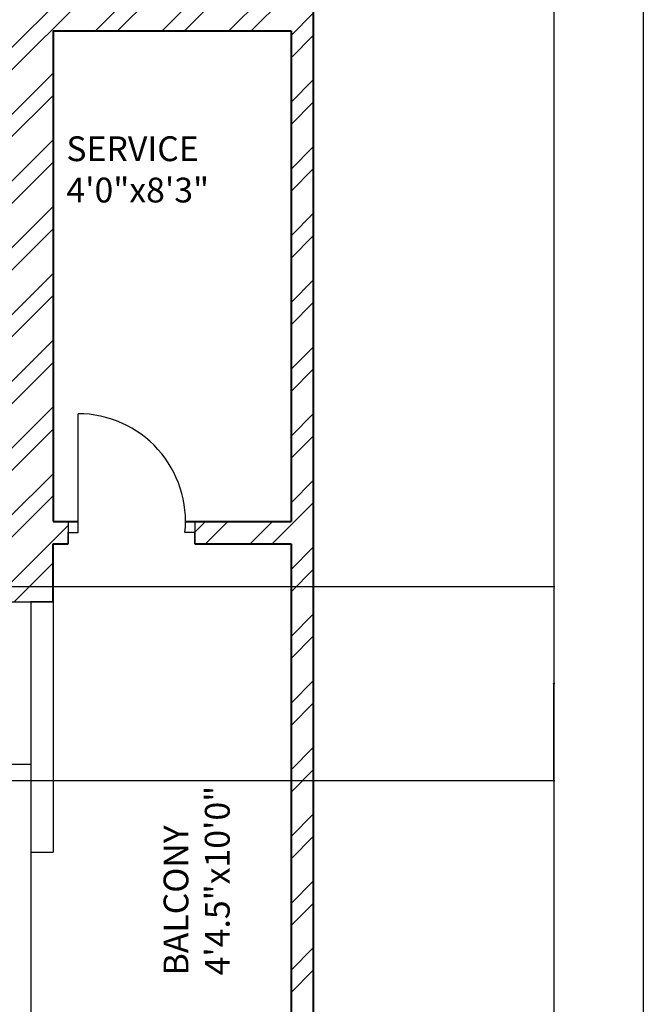
# Model space of a CAD drawing. Units: inches. Extents: x 1601 to 2297, y 1496 to 2631.
# Tile 56 of 57: x 2171 to 2297, y 2327 to 2526. Entities that reach past the tile are written whole.
import ezdxf

# ---------------------------------------------------------------- set-up
doc = ezdxf.new("R2010")
doc.units = ezdxf.units.IN
for name, color, linetype, lineweight in [('A-ANNO-DIMS', 2, 'Continuous', 18), ('A-ANNO-TTLB', 7, 'Continuous', 25), ('A-AREA-IDEN', 7, 'Continuous', 18), ('A-DOOR', 21, 'Continuous', 25), ('A-WALL', 7, 'Continuous', 40), ('A-WALL-PATT', 215, 'Continuous', 13)]:
    doc.layers.add(name, color=color, linetype=linetype, lineweight=lineweight)
doc.styles.get("Standard").update_dxf_attribs({"font": 'arial.ttf'})
doc.dimstyles.get("Standard").update_dxf_attribs({"dimtxt": 0.18, "dimasz": 0.18, "dimexe": 0.18, "dimexo": 0.0625, "dimgap": 0.09, "dimtad": 0, "dimtih": 1, "dimtoh": 1, "dimdec": 4, "dimzin": 0, "dimdsep": 46, "dimtxsty": 'Standard', "dimcen": 0.09, "dimadec": 0, "dimazin": 0, "dimtfac": 1, "dimtdec": 4, "dimtofl": 0, "dimtmove": 0, "dimatfit": 3, "dimfxl": 1, "dimtolj": 1, "dimtzin": 0, "dimarcsym": 0})

# ---------------------------------------------------------------- blocks, each defined once
blk = doc.blocks.new('*D29')
at = {"layer": 'A-ANNO-DIMS', "color": 0, "lineweight": -2, "transparency": 16777216}
for p, q in [((2230.6, 2532.33), (2279.27, 2532.33)), ((2279.09, 2532.15), (2279.09, 2084.01)), ((2279.09, 1635.51), (2279.09, 2083.64)), ((2230.6, 1635.33), (2279.27, 1635.33))]:
    blk.add_line(p, q, dxfattribs=at)
at = {"layer": 'A-ANNO-DIMS', "color": 0, "transparency": 16777216}
for points in [[(2279.06, 2532.15), (2279.12, 2532.15), (2279.09, 2532.33)], [(2279.06, 1635.51), (2279.12, 1635.51), (2279.09, 1635.33)]]:
    blk.add_solid(points, dxfattribs=at)
at = {"layer": 'Defpoints', "color": 0, "transparency": 16777216}
for p in [(2230.54, 2532.33), (2279.09, 2532.33), (2230.54, 1635.33)]:
    blk.add_point(p, dxfattribs=at)
at = {"layer": 'A-ANNO-DIMS', "color": 0, "transparency": 16777216, "insert": (2279.09, 2083.83), "char_height": 0.18, "attachment_point": 5}
blk.add_mtext('\\A1;897', dxfattribs=at)
blk = doc.blocks.new('*D51')
at = {"layer": 'A-ANNO-DIMS', "color": 0, "lineweight": -2, "transparency": 16777216}
for p, q in [((1912.15, 2411.19), (2279.27, 2411.19)), ((2279.09, 2411.01), (2279.09, 2391.83)), ((2279.09, 2372.28), (2279.09, 2391.46)), ((1912.15, 2372.1), (2279.27, 2372.1))]:
    blk.add_line(p, q, dxfattribs=at)
at = {"layer": 'A-ANNO-DIMS', "color": 0, "transparency": 16777216}
for points in [[(2279.06, 2411.01), (2279.12, 2411.01), (2279.09, 2411.19)], [(2279.06, 2372.28), (2279.12, 2372.28), (2279.09, 2372.1)]]:
    blk.add_solid(points, dxfattribs=at)
at = {"layer": 'Defpoints', "color": 0, "transparency": 16777216}
for p in [(1912.09, 2411.19), (2279.09, 2411.19), (1912.09, 2372.1)]:
    blk.add_point(p, dxfattribs=at)
at = {"layer": 'A-ANNO-DIMS', "color": 0, "transparency": 16777216, "insert": (2279.09, 2391.64), "char_height": 0.18, "attachment_point": 5}
blk.add_mtext('\\A1;39.1', dxfattribs=at)

msp = doc.modelspace()

# ---------------------------------------------------------------- hatches: boundary and pattern name
at = {"layer": 'A-WALL-PATT'}
h = msp.add_hatch(dxfattribs=at)
h.set_pattern_fill('ANSI32', color=256)
h.paths.add_polyline_path([(1842.0336, 2528.0767), (1842.0336, 2532.3254), (1686.0373, 2532.3254), (1686.0373, 2492.9493), (1695.0373, 2492.9493), (1695.0373, 2523.3254), (1827.0373, 2523.3254), (1827.0373, 2416.8254), (1834.6225, 2416.8254), (1834.6225, 2419.0754), (1834.6225, 2421.3254), (1831.5373, 2421.3254), (1831.5373, 2523.3254), (1842.0336, 2523.3254)])
h.paths.add_polyline_path([(1695.0373, 2432.9493), (1686.0373, 2432.9493), (1686.0373, 2325.989), (1695.0373, 2325.989), (1695.0373, 2347.8254), (1827.0373, 2347.8254), (1827.0373, 2287.8254), (1823.2991, 2287.8254), (1823.2991, 2283.3254), (1847.9422, 2283.3254), (1847.9422, 2285.5754), (1847.9422, 2287.8254), (1831.5373, 2287.8254), (1831.5373, 2347.8254), (1846.9946, 2347.8254), (1846.9946, 2350.0754), (1846.9946, 2352.3254), (1695.0373, 2352.3254)])
h.paths.add_polyline_path([(1807.1169, 1573.5395), (2055.0405, 1573.5395), (2055.0405, 1610.6322), (1807.1169, 1610.6322)], flags=9)
h.paths.add_polyline_path([(1841.1631, 1712.7967), (1870.3957, 1712.7967), (1870.3957, 1731.454), (1841.1631, 1731.454)], flags=9)
h.paths.add_polyline_path([(2144.3862, 1772.185), (2191.0233, 1772.185), (2191.0233, 1790.8423), (2144.3862, 1790.8423)], flags=9)
h.paths.add_polyline_path([(2143.0128, 1827.3312), (2177.9958, 1827.3312), (2177.9958, 1845.9886), (2143.0128, 1845.9886)], flags=9)
h.paths.add_polyline_path([(2041.2439, 1833.5691), (2070.8516, 1833.5691), (2070.8516, 1852.2264), (2041.2439, 1852.2264)], flags=9)
h.paths.add_polyline_path([(2097.2791, 1947.0598), (2134.2061, 1947.0598), (2134.2061, 1965.7171), (2097.2791, 1965.7171)], flags=9)
h.paths.add_polyline_path([(2214.995, 1904.3124), (2214.995, 1942.2899), (2196.3376, 1942.2899), (2196.3376, 1904.3124)], flags=9)
h.paths.add_polyline_path([(2186.6284, 2043.8031), (2219.7935, 2043.8031), (2219.7935, 2062.4605), (2186.6284, 2062.4605)], flags=9)
h.paths.add_polyline_path([(2064.0877, 2031.616), (2097.4949, 2031.616), (2097.4949, 2050.2734), (2064.0877, 2050.2734)], flags=9)
h.paths.add_polyline_path([(1973.1349, 1986.0688), (2008.4009, 1986.0688), (2008.4009, 2004.7261), (1973.1349, 2004.7261)], flags=9)
h.paths.add_polyline_path([(1976.3676, 2106.9635), (2005.7469, 2106.9635), (2005.7469, 2125.6209), (1976.3676, 2125.6209)], flags=9)
h.paths.add_polyline_path([(1991.7852, 2180.4863), (2027.0513, 2180.4863), (2027.0513, 2199.1437), (1991.7852, 2199.1437)], flags=9)
h.paths.add_polyline_path([(2106.1801, 2187.9359), (2152.2101, 2187.9359), (2152.2101, 2206.5932), (2106.1801, 2206.5932)], flags=9)
h.paths.add_polyline_path([(2148.6686, 2262.2542), (2182.318, 2262.2542), (2182.318, 2280.9115), (2148.6686, 2280.9115)], flags=9)
h.paths.add_polyline_path([(2041.6327, 2252.8147), (2071.2405, 2252.8147), (2071.2405, 2271.4721), (2041.6327, 2271.4721)], flags=9)
h.paths.add_polyline_path([(2063.9734, 2375.4265), (2100.9004, 2375.4265), (2100.9004, 2394.0839), (2063.9734, 2394.0839)], flags=9)
h.paths.add_polyline_path([(2216.4955, 2330.9748), (2216.4955, 2370.2654), (2197.8381, 2370.2654), (2197.8381, 2330.9748)], flags=9)
h.paths.add_polyline_path([(2179.1416, 2485.8687), (2212.3067, 2485.8687), (2212.3067, 2504.5261), (2179.1416, 2504.5261)], flags=9)
h.paths.add_polyline_path([(2078.7442, 2471.1516), (2112.1514, 2471.1516), (2112.1514, 2489.809), (2078.7442, 2489.809)], flags=9)
h.paths.add_polyline_path([(1915.9631, 2329.4668), (1952.8902, 2329.4668), (1952.8902, 2348.1241), (1915.9631, 2348.1241)], flags=9)
h.paths.add_polyline_path([(1904.3189, 2499.6709), (1940.4512, 2499.6709), (1940.4512, 2518.3282), (1904.3189, 2518.3282)], flags=9)
h.paths.add_polyline_path([(1892.3665, 2100.4595), (1925.6374, 2100.4595), (1925.6374, 2119.1169), (1892.3665, 2119.1169)], flags=9)
h.paths.add_polyline_path([(1909.2984, 1805.9631), (1946.2254, 1805.9631), (1946.2254, 1824.6205), (1909.2984, 1824.6205)], flags=9)
h.paths.add_polyline_path([(1934.6056, 1658.616), (1970.738, 1658.616), (1970.738, 1677.2733), (1934.6056, 1677.2733)], flags=9)
h.paths.add_polyline_path([(1711.2052, 1789.8902), (1750.0456, 1789.8902), (1750.0456, 1808.5476), (1711.2052, 1808.5476)], flags=9)
h.paths.add_polyline_path([(1742.7874, 1854.6743), (1771.9449, 1854.6743), (1771.9449, 1873.3317), (1742.7874, 1873.3317)], flags=9)
h.paths.add_polyline_path([(1807.3592, 1997.7912), (1850.1116, 1997.7912), (1850.1116, 2016.4486), (1807.3592, 2016.4486)], flags=9)
h.paths.add_polyline_path([(1717.4579, 2237.7844), (1760.2103, 2237.7844), (1760.2103, 2256.4417), (1717.4579, 2256.4417)], flags=9)
h.paths.add_polyline_path([(1780.9285, 2324.0623), (1810.086, 2324.0623), (1810.086, 2342.7197), (1780.9285, 2342.7197)], flags=25)
h.paths.add_polyline_path([(1837.696, 2449.2024), (1866.9286, 2449.2024), (1866.9286, 2467.8598), (1837.696, 2467.8598)], flags=9)
h.paths.add_polyline_path([(1712.7752, 2484.9404), (1751.6156, 2484.9404), (1751.6156, 2503.5977), (1712.7752, 2503.5977)], flags=25)
h = msp.add_hatch(dxfattribs=at)
h.set_pattern_fill('ANSI32', color=256)
h.paths.add_polyline_path([(2230.5373, 2532.3254), (2106.0595, 2532.3254), (2106.0595, 2523.3254), (2169.0373, 2523.3254), (2169.0373, 2424.3254), (2091.3989, 2424.3254), (2091.3989, 2419.8254), (2169.0373, 2419.8254), (2169.0373, 2408.1385), (2178.0373, 2408.1385), (2178.0373, 2419.8254), (2181.0581, 2419.8254), (2181.0581, 2422.0754), (2181.0581, 2424.3254), (2178.0373, 2424.3254), (2178.0373, 2523.3254), (2226.0373, 2523.3254), (2226.0373, 2424.3254), (2206.6251, 2424.3254), (2206.6251, 2419.8254), (2226.0373, 2419.8254), (2226.0373, 2299.8254), (2226.0373, 2295.3254), (2178.0373, 2295.3254), (2178.0373, 2312.1385), (2169.0373, 2312.1385), (2169.0373, 2295.3254), (2130.0373, 2295.3254), (2130.0373, 2279.1364), (2128.0593, 2279.1364), (2128.0593, 2274.6364), (2130.0373, 2274.6364), (2130.0373, 2260.7505), (2134.5373, 2260.7505), (2134.5373, 2290.8254), (2226.0373, 2290.8254), (2226.0373, 2279.2475), (2230.5373, 2279.2475), (2230.5373, 2347.8254)])
h.paths.add_polyline_path([(2070.0595, 2532.3254), (2031.0373, 2532.3254), (2031.0373, 2466.3254), (2003.9878, 2466.3254), (2003.9878, 2457.3254), (2031.0373, 2457.3254), (2031.0373, 2419.8254), (2031.0373, 2373.1914), (2035.5373, 2373.1914), (2035.5373, 2419.8254), (2047.3393, 2419.8254), (2047.3393, 2424.3254), (2035.5373, 2424.3254), (2035.5373, 2523.3254), (2070.0595, 2523.3254), (2070.0595, 2527.8254)])
h.paths.add_polyline_path([(1893.0373, 2532.3254), (1866.0336, 2532.3254), (1866.0336, 2523.3254), (1888.5373, 2523.3254), (1888.5373, 2347.8254), (1893.0373, 2347.8254), (1893.0373, 2457.3254), (1907.9878, 2457.3254), (1907.9878, 2466.3254), (1893.0373, 2466.3254)])
h = msp.add_hatch(dxfattribs=at)
h.set_pattern_fill('ANSI32', color=256)
h.paths.add_polyline_path([(1973.9371, 2211.3254), (1893.0373, 2211.3254), (1893.0373, 2287.8254), (1884.6167, 2287.8254), (1884.6167, 2285.5754), (1884.6167, 2283.3254), (1888.5373, 2283.3254), (1888.5373, 2145.3254), (1695.0373, 2145.3254), (1695.0373, 2173.8724), (1690.5373, 2173.8724), (1686.0373, 2173.8724), (1686.0373, 2136.3254), (1722.5687, 2136.3254), (1722.5687, 2117.4352), (1731.5687, 2117.4352), (1731.5687, 2136.3254), (1893.0373, 2136.3254), (1893.0373, 2202.3254), (1959.0373, 2202.3254), (1959.0373, 2182.1303), (1968.0373, 2182.1303), (1968.0373, 2202.3254), (1973.9371, 2202.3254)])
h.paths.add_polyline_path([(2094.0373, 2274.6364), (2096.4294, 2274.6364), (2096.4294, 2276.8864), (2096.4294, 2279.1364), (2094.0373, 2279.1364), (2094.0373, 2290.8254), (2094.0373, 2295.3254), (2089.5373, 2295.3254), (2089.5373, 2230.8254), (2035.5373, 2230.8254), (2035.5373, 2299.8254), (2031.0373, 2299.8254), (2031.0373, 2211.3254), (2023.0065, 2211.3254), (2023.0065, 2202.3254), (2031.0373, 2202.3254), (2031.0373, 2140.8254), (1968.0373, 2140.8254), (1968.0373, 2145.9106), (1963.5373, 2145.9106), (1959.0373, 2145.9106), (1959.0373, 2116.839), (1963.5373, 2116.839), (1968.0373, 2116.839), (1968.0373, 2131.8254), (2031.0373, 2131.8254), (2031.0373, 2094.3254), (2031.0373, 2085.3254), (2031.0373, 2056.8254), (1968.0373, 2056.8254), (1968.0373, 2070.4947), (1963.5373, 2070.4947), (1959.0373, 2070.4947), (1959.0373, 2040.3029), (1968.0373, 2040.3029), (1968.0373, 2047.8254), (2031.0373, 2047.8254), (2031.0373, 1983.3254), (2031.0373, 1978.8254), (2021.1979, 1978.8254), (2021.1979, 1974.3254), (2031.0373, 1974.3254), (2031.0373, 1954.3528), (2035.5373, 1954.3528), (2035.5373, 1974.3254), (2035.5373, 1981.8254), (2055.5513, 1981.8254), (2055.5513, 1986.3254), (2035.5373, 1986.3254), (2035.5373, 2047.8254), (2040.0373, 2047.8254), (2040.0373, 2085.3254), (2040.0373, 2094.3254), (2040.0373, 2140.8254), (2035.5373, 2140.8254), (2035.5373, 2226.3254), (2089.5373, 2226.3254), (2094.0373, 2226.3254)])
h.paths.add_polyline_path([(2226.0373, 2230.8254), (2134.5373, 2230.8254), (2134.5373, 2233.5437), (2130.0373, 2233.5437), (2130.0373, 2226.3254), (2134.5373, 2226.3254), (2226.0373, 2226.3254)])
h.paths.add_polyline_path([(1807.1169, 1573.5395), (2055.0405, 1573.5395), (2055.0405, 1610.6322), (1807.1169, 1610.6322)], flags=9)
h.paths.add_polyline_path([(1841.1631, 1712.7967), (1870.3957, 1712.7967), (1870.3957, 1731.454), (1841.1631, 1731.454)], flags=9)
h.paths.add_polyline_path([(2144.3862, 1772.185), (2191.0233, 1772.185), (2191.0233, 1790.8423), (2144.3862, 1790.8423)], flags=9)
h.paths.add_polyline_path([(2143.0128, 1827.3312), (2177.9958, 1827.3312), (2177.9958, 1845.9886), (2143.0128, 1845.9886)], flags=9)
h.paths.add_polyline_path([(2041.2439, 1833.5691), (2070.8516, 1833.5691), (2070.8516, 1852.2264), (2041.2439, 1852.2264)], flags=9)
h.paths.add_polyline_path([(2097.2791, 1947.0598), (2134.2061, 1947.0598), (2134.2061, 1965.7171), (2097.2791, 1965.7171)], flags=9)
h.paths.add_polyline_path([(2214.995, 1904.3124), (2214.995, 1942.2899), (2196.3376, 1942.2899), (2196.3376, 1904.3124)], flags=9)
h.paths.add_polyline_path([(2186.6284, 2043.8031), (2219.7935, 2043.8031), (2219.7935, 2062.4605), (2186.6284, 2062.4605)], flags=9)
h.paths.add_polyline_path([(2064.0877, 2031.616), (2097.4949, 2031.616), (2097.4949, 2050.2734), (2064.0877, 2050.2734)], flags=9)
h.paths.add_polyline_path([(1973.1349, 1986.0688), (2008.4009, 1986.0688), (2008.4009, 2004.7261), (1973.1349, 2004.7261)], flags=25)
h.paths.add_polyline_path([(1976.3676, 2106.9635), (2005.7469, 2106.9635), (2005.7469, 2125.6209), (1976.3676, 2125.6209)], flags=25)
h.paths.add_polyline_path([(1991.7852, 2180.4863), (2027.0513, 2180.4863), (2027.0513, 2199.1437), (1991.7852, 2199.1437)], flags=25)
h.paths.add_polyline_path([(2106.1801, 2187.9359), (2152.2101, 2187.9359), (2152.2101, 2206.5932), (2106.1801, 2206.5932)], flags=9)
h.paths.add_polyline_path([(2148.6686, 2262.2542), (2182.318, 2262.2542), (2182.318, 2280.9115), (2148.6686, 2280.9115)], flags=9)
h.paths.add_polyline_path([(2041.6327, 2252.8147), (2071.2405, 2252.8147), (2071.2405, 2271.4721), (2041.6327, 2271.4721)], flags=25)
h.paths.add_polyline_path([(2063.9734, 2375.4265), (2100.9004, 2375.4265), (2100.9004, 2394.0839), (2063.9734, 2394.0839)], flags=9)
h.paths.add_polyline_path([(2216.4955, 2330.9748), (2216.4955, 2370.2654), (2197.8381, 2370.2654), (2197.8381, 2330.9748)], flags=9)
h.paths.add_polyline_path([(2179.1416, 2485.8687), (2212.3067, 2485.8687), (2212.3067, 2504.5261), (2179.1416, 2504.5261)], flags=9)
h.paths.add_polyline_path([(2078.7442, 2471.1516), (2112.1514, 2471.1516), (2112.1514, 2489.809), (2078.7442, 2489.809)], flags=9)
h.paths.add_polyline_path([(1915.9631, 2329.4668), (1952.8902, 2329.4668), (1952.8902, 2348.1241), (1915.9631, 2348.1241)], flags=9)
h.paths.add_polyline_path([(1904.3189, 2499.6709), (1940.4512, 2499.6709), (1940.4512, 2518.3282), (1904.3189, 2518.3282)], flags=9)
h.paths.add_polyline_path([(1892.3665, 2100.4595), (1925.6374, 2100.4595), (1925.6374, 2119.1169), (1892.3665, 2119.1169)], flags=9)
h.paths.add_polyline_path([(1909.2984, 1805.9631), (1946.2254, 1805.9631), (1946.2254, 1824.6205), (1909.2984, 1824.6205)], flags=9)
h.paths.add_polyline_path([(1934.6056, 1658.616), (1970.738, 1658.616), (1970.738, 1677.2733), (1934.6056, 1677.2733)], flags=9)
h.paths.add_polyline_path([(1711.2052, 1789.8902), (1750.0456, 1789.8902), (1750.0456, 1808.5476), (1711.2052, 1808.5476)], flags=9)
h.paths.add_polyline_path([(1742.7874, 1854.6743), (1771.9449, 1854.6743), (1771.9449, 1873.3317), (1742.7874, 1873.3317)], flags=9)
h.paths.add_polyline_path([(1807.3592, 1997.7912), (1850.1116, 1997.7912), (1850.1116, 2016.4486), (1807.3592, 2016.4486)], flags=9)
h.paths.add_polyline_path([(1717.4579, 2237.7844), (1760.2103, 2237.7844), (1760.2103, 2256.4417), (1717.4579, 2256.4417)], flags=25)
h.paths.add_polyline_path([(1780.9285, 2324.0623), (1810.086, 2324.0623), (1810.086, 2342.7197), (1780.9285, 2342.7197)], flags=9)
h.paths.add_polyline_path([(1837.696, 2449.2024), (1866.9286, 2449.2024), (1866.9286, 2467.8598), (1837.696, 2467.8598)], flags=9)
h.paths.add_polyline_path([(1712.7752, 2484.9404), (1751.6156, 2484.9404), (1751.6156, 2503.5977), (1712.7752, 2503.5977)], flags=9)
h = msp.add_hatch(dxfattribs=at)
h.set_pattern_fill('ANSI32', color=256)
h.paths.add_polyline_path([(2230.5373, 1861.8254), (2182.5373, 1861.8254), (2182.5373, 1885.3637), (2178.0373, 1885.3637), (2178.0373, 1861.8254), (2166.0373, 1861.8254), (2134.5373, 1861.8254), (2130.0373, 1861.8254), (2130.0373, 1841.4682), (2126.8833, 1841.4682), (2126.8833, 1836.9682), (2130.0373, 1836.9682), (2130.0373, 1822.7302), (2134.5373, 1822.7302), (2134.5373, 1857.3254), (2166.0373, 1857.3254), (2226.0373, 1857.3254), (2226.0373, 1846.1155), (2230.5373, 1846.1155)])
h.paths.add_polyline_path([(2226.0373, 1797.3254), (2134.5373, 1797.3254), (2134.5373, 1800.6636), (2132.2873, 1800.6636), (2130.0373, 1800.6636), (2130.0373, 1797.3254), (2130.0373, 1792.8254), (2167.7264, 1792.8254), (2226.0373, 1792.8254)])
h.paths.add_polyline_path([(2230.5373, 1822.1155), (2226.0373, 1822.1155), (2226.0373, 1760.8563), (2230.5373, 1760.8563)])
h.paths.add_polyline_path([(2230.5373, 1700.8563), (2226.0373, 1700.8563), (2226.0373, 1644.3254), (2140.2517, 1644.3254), (2140.2517, 1635.3254), (2230.5373, 1635.3254)])
h.paths.add_polyline_path([(2080.2517, 1639.8254), (2080.2517, 1644.3254), (2035.5373, 1644.3254), (2035.5373, 1792.8254), (2094.0373, 1792.8254), (2094.0373, 1797.3254), (2094.0373, 1836.9682), (2097.1057, 1836.9682), (2097.1057, 1839.2182), (2097.1057, 1841.4682), (2094.0373, 1841.4682), (2094.0373, 1862.2276), (2089.5373, 1862.2276), (2089.5373, 1797.3254), (2035.5373, 1797.3254), (2035.5373, 1857.3254), (2035.5373, 1885.0916), (2031.0373, 1885.0916), (2031.0373, 1710.3254), (2012.329, 1710.3254), (2012.329, 1701.3254), (2031.0373, 1701.3254), (2031.0373, 1644.3254), (2031.0373, 1635.3254), (2080.2517, 1635.3254)])
h.paths.add_polyline_path([(1836.0373, 1653.2033), (1842.6171, 1653.2033), (1842.6171, 1657.7033), (1842.6171, 1662.2033), (1831.5373, 1662.2033), (1831.5373, 1764.2033), (1835.3881, 1764.2033), (1835.3881, 1766.4533), (1835.3881, 1768.7033), (1831.5373, 1768.7033), (1827.0373, 1768.7033), (1827.0373, 1662.2033), (1827.0373, 1635.3254), (1836.0373, 1635.3254)])
h.paths.add_polyline_path([(1893.0373, 1701.3254), (1907.193, 1701.3254), (1907.193, 1705.8254), (1907.193, 1710.3254), (1893.0373, 1710.3254), (1893.0373, 1819.8254), (1882.6444, 1819.8254), (1882.6444, 1817.5754), (1882.6444, 1815.3254), (1888.5373, 1815.3254), (1888.5373, 1662.2033), (1884.0373, 1662.2033), (1866.6171, 1662.2033), (1866.6171, 1653.2033), (1882.391, 1653.2033), (1884.0373, 1653.2033), (1884.0373, 1635.3254), (1893.0373, 1635.3254)])
h.paths.add_polyline_path([(1739.3335, 1639.8254), (1739.3335, 1644.3254), (1695.0373, 1644.3254), (1695.0373, 1702.0135), (1690.5373, 1702.0135), (1686.0373, 1702.0135), (1686.0373, 1635.3254), (1739.3335, 1635.3254)])
h.paths.add_polyline_path([(1827.0373, 1644.3254), (1799.3335, 1644.3254), (1799.3335, 1635.3254), (1827.0373, 1635.3254)])
h.paths.add_polyline_path([(1695.0373, 1815.3254), (1849.2759, 1815.3254), (1849.2759, 1819.8254), (1807.5373, 1819.8254), (1807.5373, 1879.8254), (1851.1533, 1879.8254), (1851.1533, 1882.0754), (1851.1533, 1884.3254), (1799.3405, 1884.3254), (1799.3405, 1882.0754), (1799.3405, 1879.8254), (1803.0373, 1879.8254), (1803.0373, 1819.8254), (1695.0373, 1819.8254), (1695.0373, 1835.0458), (1690.5373, 1835.0458), (1686.0373, 1835.0458), (1686.0373, 1766.1753), (1695.0373, 1766.1753)])
h.paths.add_polyline_path([(1775.8157, 1884.3254), (1695.0373, 1884.3254), (1695.0373, 1912.9526), (1690.5373, 1912.9526), (1686.0373, 1912.9526), (1686.0373, 1859.0458), (1695.0373, 1859.0458), (1695.0373, 1879.8254), (1775.8157, 1879.8254)])
h.paths.add_polyline_path([(1893.0373, 2031.3254), (1731.5687, 2031.3254), (1731.5687, 2057.4352), (1722.5687, 2057.4352), (1722.5687, 2031.3254), (1686.0373, 2031.3254), (1686.0373, 1972.9526), (1695.0373, 1972.9526), (1695.0373, 2022.3254), (1888.5373, 2022.3254), (1888.5373, 1884.3254), (1883.4996, 1884.3254), (1883.4996, 1879.8254), (1893.0373, 1879.8254), (1893.0373, 1974.3254), (1976.6199, 1974.3254), (1976.6199, 1978.8254), (1968.0373, 1978.8254), (1968.0373, 1983.3254), (1968.0373, 2008.4756), (1963.5373, 2008.4756), (1959.0373, 2008.4756), (1959.0373, 1983.3254), (1893.0373, 1983.3254)])
h.paths.add_polyline_path([(2230.5373, 2140.4745), (2226.0373, 2140.4745), (2226.0373, 2094.3254), (2040.0373, 2094.3254), (2040.0373, 2085.3254), (2178.0373, 2085.3254), (2178.0373, 2065.6965), (2182.5373, 2065.6965), (2182.5373, 2085.3254), (2226.0373, 2085.3254), (2226.0373, 1986.3254), (2211.2679, 1986.3254), (2211.2679, 1981.8254), (2230.5373, 1981.8254)])
h.paths.add_polyline_path([(2187.6292, 1986.3254), (2182.5373, 1986.3254), (2182.5373, 2029.6965), (2178.0373, 2029.6965), (2178.0373, 1986.3254), (2099.05, 1986.3254), (2099.05, 1981.8254), (2178.0373, 1981.8254), (2178.0373, 1969.3637), (2182.5373, 1969.3637), (2182.5373, 1981.8254), (2187.6292, 1981.8254), (2187.6292, 1984.0754)])
h.paths.add_polyline_path([(1807.1169, 1573.5395), (2055.0405, 1573.5395), (2055.0405, 1610.6322), (1807.1169, 1610.6322)], flags=9)
h.paths.add_polyline_path([(1841.1631, 1712.7967), (1870.3957, 1712.7967), (1870.3957, 1731.454), (1841.1631, 1731.454)], flags=9)
h.paths.add_polyline_path([(2144.3862, 1772.185), (2191.0233, 1772.185), (2191.0233, 1790.8423), (2144.3862, 1790.8423)], flags=9)
h.paths.add_polyline_path([(2143.0128, 1827.3312), (2177.9958, 1827.3312), (2177.9958, 1845.9886), (2143.0128, 1845.9886)], flags=25)
h.paths.add_polyline_path([(2041.2439, 1833.5691), (2070.8516, 1833.5691), (2070.8516, 1852.2264), (2041.2439, 1852.2264)], flags=25)
h.paths.add_polyline_path([(2097.2791, 1947.0598), (2134.2061, 1947.0598), (2134.2061, 1965.7171), (2097.2791, 1965.7171)], flags=9)
h.paths.add_polyline_path([(2214.995, 1904.3124), (2214.995, 1942.2899), (2196.3376, 1942.2899), (2196.3376, 1904.3124)], flags=9)
h.paths.add_polyline_path([(2186.6284, 2043.8031), (2219.7935, 2043.8031), (2219.7935, 2062.4605), (2186.6284, 2062.4605)], flags=25)
h.paths.add_polyline_path([(2064.0877, 2031.616), (2097.4949, 2031.616), (2097.4949, 2050.2734), (2064.0877, 2050.2734)], flags=25)
h.paths.add_polyline_path([(1973.1349, 1986.0688), (2008.4009, 1986.0688), (2008.4009, 2004.7261), (1973.1349, 2004.7261)], flags=9)
h.paths.add_polyline_path([(1976.3676, 2106.9635), (2005.7469, 2106.9635), (2005.7469, 2125.6209), (1976.3676, 2125.6209)], flags=9)
h.paths.add_polyline_path([(1991.7852, 2180.4863), (2027.0513, 2180.4863), (2027.0513, 2199.1437), (1991.7852, 2199.1437)], flags=9)
h.paths.add_polyline_path([(2106.1801, 2187.9359), (2152.2101, 2187.9359), (2152.2101, 2206.5932), (2106.1801, 2206.5932)], flags=9)
h.paths.add_polyline_path([(2148.6686, 2262.2542), (2182.318, 2262.2542), (2182.318, 2280.9115), (2148.6686, 2280.9115)], flags=9)
h.paths.add_polyline_path([(2041.6327, 2252.8147), (2071.2405, 2252.8147), (2071.2405, 2271.4721), (2041.6327, 2271.4721)], flags=9)
h.paths.add_polyline_path([(2063.9734, 2375.4265), (2100.9004, 2375.4265), (2100.9004, 2394.0839), (2063.9734, 2394.0839)], flags=9)
h.paths.add_polyline_path([(2216.4955, 2330.9748), (2216.4955, 2370.2654), (2197.8381, 2370.2654), (2197.8381, 2330.9748)], flags=9)
h.paths.add_polyline_path([(2179.1416, 2485.8687), (2212.3067, 2485.8687), (2212.3067, 2504.5261), (2179.1416, 2504.5261)], flags=9)
h.paths.add_polyline_path([(2078.7442, 2471.1516), (2112.1514, 2471.1516), (2112.1514, 2489.809), (2078.7442, 2489.809)], flags=9)
h.paths.add_polyline_path([(1915.9631, 2329.4668), (1952.8902, 2329.4668), (1952.8902, 2348.1241), (1915.9631, 2348.1241)], flags=9)
h.paths.add_polyline_path([(1904.3189, 2499.6709), (1940.4512, 2499.6709), (1940.4512, 2518.3282), (1904.3189, 2518.3282)], flags=9)
h.paths.add_polyline_path([(1892.3665, 2100.4595), (1925.6374, 2100.4595), (1925.6374, 2119.1169), (1892.3665, 2119.1169)], flags=9)
h.paths.add_polyline_path([(1909.2984, 1805.9631), (1946.2254, 1805.9631), (1946.2254, 1824.6205), (1909.2984, 1824.6205)], flags=9)
h.paths.add_polyline_path([(1934.6056, 1658.616), (1970.738, 1658.616), (1970.738, 1677.2733), (1934.6056, 1677.2733)], flags=9)
h.paths.add_polyline_path([(1711.2052, 1789.8902), (1750.0456, 1789.8902), (1750.0456, 1808.5476), (1711.2052, 1808.5476)], flags=25)
h.paths.add_polyline_path([(1742.7874, 1854.6743), (1771.9449, 1854.6743), (1771.9449, 1873.3317), (1742.7874, 1873.3317)], flags=25)
h.paths.add_polyline_path([(1807.3592, 1997.7912), (1850.1116, 1997.7912), (1850.1116, 2016.4486), (1807.3592, 2016.4486)], flags=25)
h.paths.add_polyline_path([(1717.4579, 2237.7844), (1760.2103, 2237.7844), (1760.2103, 2256.4417), (1717.4579, 2256.4417)], flags=9)
h.paths.add_polyline_path([(1780.9285, 2324.0623), (1810.086, 2324.0623), (1810.086, 2342.7197), (1780.9285, 2342.7197)], flags=9)
h.paths.add_polyline_path([(1837.696, 2449.2024), (1866.9286, 2449.2024), (1866.9286, 2467.8598), (1837.696, 2467.8598)], flags=9)
h.paths.add_polyline_path([(1712.7752, 2484.9404), (1751.6156, 2484.9404), (1751.6156, 2503.5977), (1712.7752, 2503.5977)], flags=9)

# ---------------------------------------------------------------- linework, layer by layer
at = {"layer": 'A-ANNO-TTLB'}
msp.add_lwpolyline([(1600.5933, 2631.1477), (2297.129, 2631.1477), (2297.129, 1496.1026), (1600.5933, 1496.1026)], close=True, dxfattribs=at)
at = {"layer": 'A-DOOR'}
for p, q in [((2183.0581, 2422.0754), (2183.0581, 2446.0754)), ((2181.0581, 2424.3254), (2181.0581, 2419.8254)), ((2206.6251, 2424.3254), (2206.6251, 2419.8254)), ((2181.0581, 2419.8254), (2181.0581, 2422.0754)), ((2181.0581, 2422.0754), (2183.0581, 2422.0754)), ((2206.6251, 2422.0754), (2204.6251, 2422.0754)), ((2206.6251, 2419.8254), (2206.6251, 2422.0754)), ((2169.0373, 2408.1385), (2178.0373, 2408.1385)), ((2178.0373, 2408.1385), (2173.5373, 2408.1385)), ((2173.5373, 2408.1385), (2173.5373, 2348.1385)), ((2178.0373, 2408.1385), (2178.0373, 2357.5835)), ((2169.0373, 2375.3908), (2173.5373, 2375.3908)), ((2173.5373, 2357.5835), (2178.0373, 2357.5835)), ((2173.5373, 2348.1385), (2173.5373, 2312.1385))]:
    msp.add_line(p, q, dxfattribs=at)
msp.add_arc((2183.0581, 2424.385), 21.6903, 353.887391, 90, dxfattribs=at)
at = {"layer": 'A-WALL'}
for p, q in [((2230.5373, 2532.3254), (2230.5373, 2347.8254)), ((2178.0373, 2523.3254), (2178.0373, 2424.3254)), ((2178.0373, 2523.3254), (2226.0373, 2523.3254)), ((2226.0373, 2523.3254), (2226.0373, 2424.3254)), ((2178.0373, 2424.3254), (2183.0581, 2424.3254)), ((2204.7483, 2424.3254), (2226.0373, 2424.3254)), ((2178.0373, 2419.8254), (2181.0581, 2419.8254)), ((2178.0373, 2408.1385), (2178.0373, 2419.8254)), ((2206.6251, 2419.8254), (2226.0373, 2419.8254)), ((2226.0373, 2419.8254), (2226.0373, 2352.3254)), ((2226.0373, 2419.8254), (2226.0373, 2299.8254)), ((2226.0373, 2352.3254), (2226.0373, 2299.8254)), ((2230.5373, 2347.8254), (2230.5373, 2279.2475))]:
    msp.add_line(p, q, dxfattribs=at)

# ---------------------------------------------------------------- texts
at = {"layer": 'A-AREA-IDEN', "insert": (2180.7054, 2502.038), "char_height": 5, "attachment_point": 1}
msp.add_mtext_dynamic_manual_height_columns('SERVICE\\P4\'0"x8\'3"', width=45.331959, gutter_width=12.5, heights=[0], dxfattribs=at)
at = {"layer": 'A-AREA-IDEN', "insert": (2200.3228, 2332.7364), "char_height": 5, "attachment_point": 1, "rotation": 90}
msp.add_mtext_dynamic_manual_height_columns('BALCONY\\P4\'4.5"x10\'0"', width=40.44844, gutter_width=12.5, heights=[0], dxfattribs=at)

# ---------------------------------------------------------------- dimensions: what is measured, and where the dimension line sits
at = {"layer": 'A-ANNO-DIMS'}
for base, p1, p2, override, picture, middle in [((2279.0873, 2532.3254), (2230.5373, 1635.3254), (2230.5373, 2532.3254), {"dimdec": 0, "dimlfac": 1, "dimrnd": 0, "dimzin": 0, "dimdsep": 46, "dimlunit": 2}, '*D29', (2279.0873, 2083.8254)), ((2279.0873, 2411.1939), (1912.0896, 2372.0953), (1912.0896, 2411.1939), {"dimdec": 1, "dimlfac": 1, "dimrnd": 0, "dimzin": 0, "dimdsep": 46, "dimlunit": 2}, '*D51', (2279.0873, 2391.6446))]:
    dim = msp.add_linear_dim(base=base, p1=p1, p2=p2, angle=90, dimstyle='Standard', override=override, dxfattribs=at)
    dim.commit()
    dim.dimension.update_dxf_attribs({"geometry": picture, "text_midpoint": middle})

doc.saveas('drawing.dxf')
